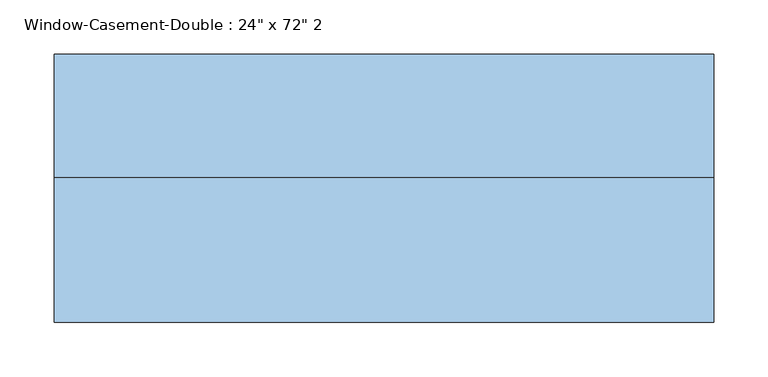
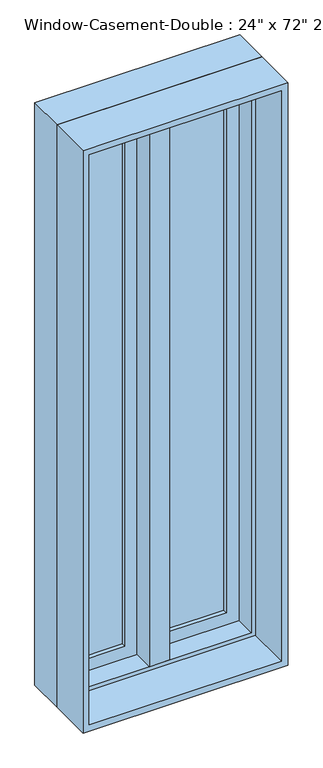
"""IFC4 building model written with IfcOpenShell, lengths in millimetres: window geometry."""

from ifc_helpers import new_model, si_unit, frame, origin, place, context, project, spatial, polyline, outline, extrude, faceted_brep, source, transform, mapped, element, save


def window_0389f97f(model_context):
    return source(origin(), model_context, "Body", "SolidModel", [
        faceted_brep([(9.525, 133.35, 2730.5), (-9.525, 133.35, 2730.5), (-9.525, 82.55, 2730.5), (9.525, 82.55, 2730.5), (9.525, 133.35, 927.1), (9.525, 82.55, 927.1), (-9.525, 82.55, 927.1), (-9.525, 133.35, 927.1), (-9.525, 82.55, 946.15), (-9.525, 82.55, 2711.45), (-30.1625, 82.55, 946.15), (-30.1625, 82.55, 2711.45), (-30.1625, 19.05, 946.15), (-30.1625, 19.05, 2711.45), (30.1625, 19.05, 946.15), (30.1625, 19.05, 2711.45), (30.1625, 82.55, 946.15), (30.1625, 82.55, 2711.45), (9.525, 82.55, 946.15), (9.525, 82.55, 2711.45)], [[[0, 1, 2, 3]], [[4, 5, 6, 7]], [[1, 0, 4, 7]], [[2, 1, 7, 6, 8, 9]], [[9, 8, 10, 11]], [[11, 10, 12, 13]], [[13, 12, 14, 15]], [[15, 14, 16, 17]], [[17, 16, 18, 19]], [[0, 3, 19, 18, 5, 4]], [[18, 8, 6, 5]], [[9, 19, 3, 2]], [[8, 18, 16, 14, 12, 10]], [[19, 9, 11, 13, 15, 17]]]),
        extrude(outline(polyline([(-66.675, 114.3), (-66.675, 107.95), (-234.95, 107.95), (-234.95, 114.3), (-66.675, 114.3)])), frame((0.0, 0.0, 984.25), z_axis=(0.0, 0.0, 1.0), x_axis=(1.0, 0.0, 0.0)), (0.0, 0.0, 1.0), 1689.1),
        extrude(outline(polyline([(-234.95, 95.25), (-234.95, 101.6), (-66.675, 101.6), (-66.675, 95.25), (-234.95, 95.25)])), frame((0.0, 0.0, 984.25), z_axis=(0.0, 0.0, 1.0), x_axis=(1.0, 0.0, 0.0)), (0.0, 0.0, 1.0), 1689.1),
        extrude(outline(polyline([(234.95, 114.3), (234.95, 107.95), (66.675, 107.95), (66.675, 114.3), (234.95, 114.3)])), frame((0.0, 0.0, 984.25), z_axis=(0.0, 0.0, 1.0), x_axis=(1.0, 0.0, 0.0)), (0.0, 0.0, 1.0), 1689.1),
        extrude(outline(polyline([(66.675, 95.25), (66.675, 101.6), (234.95, 101.6), (234.95, 95.25), (66.675, 95.25)])), frame((0.0, 0.0, 984.25), z_axis=(0.0, 0.0, 1.0), x_axis=(1.0, 0.0, 0.0)), (0.0, 0.0, 1.0), 1689.1),
        extrude(outline(polyline([(2730.5, -292.1), (927.1, -292.1), (927.1, -9.525), (2730.5, -9.525), (2730.5, -292.1)]), holes=[polyline([(2673.35, -66.675), (984.25, -66.675), (984.25, -234.95), (2673.35, -234.95), (2673.35, -66.675)])]), frame((0.0, 82.55, 0.0), z_axis=(0.0, 1.0, 0.0), x_axis=(0.0, 0.0, 1.0)), (0.0, 0.0, 1.0), 44.45),
        extrude(outline(polyline([(927.1, 292.1), (2730.5, 292.1), (2730.5, 9.525), (927.1, 9.525), (927.1, 292.1)]), holes=[polyline([(984.25, 66.675), (2673.35, 66.675), (2673.35, 234.95), (984.25, 234.95), (984.25, 66.675)])]), frame((0.0, 82.55, 0.0), z_axis=(0.0, 1.0, 0.0), x_axis=(0.0, 0.0, 1.0)), (0.0, 0.0, 1.0), 44.45),
        extrude(outline(polyline([(2743.2, -304.8), (914.4, -304.8), (914.4, 304.8), (2743.2, 304.8), (2743.2, -304.8)]), holes=[polyline([(2724.15, 285.75), (933.45, 285.75), (933.45, -285.75), (2724.15, -285.75), (2724.15, 285.75)])]), frame((0.0, -114.3, 0.0), z_axis=(0.0, 1.0, 0.0), x_axis=(0.0, 0.0, 1.0)), (0.0, 0.0, 1.0), 133.35),
        faceted_brep([(273.05, 82.55, 2711.45), (273.05, 19.05, 2711.45), (-273.05, 19.05, 2711.45), (-273.05, 82.55, 2711.45), (292.1, 133.35, 2730.5), (292.1, 82.55, 2730.5), (-292.1, 82.55, 2730.5), (-292.1, 133.35, 2730.5), (304.8, 19.05, 2743.2), (304.8, 133.35, 2743.2), (-304.8, 133.35, 2743.2), (-304.8, 19.05, 2743.2), (-273.05, 19.05, 946.15), (-273.05, 82.55, 946.15), (-292.1, 82.55, 927.1), (-292.1, 133.35, 927.1), (-304.8, 133.35, 914.4), (-304.8, 19.05, 914.4), (273.05, 19.05, 946.15), (273.05, 82.55, 946.15), (292.1, 82.55, 927.1), (292.1, 133.35, 927.1), (304.8, 133.35, 914.4), (304.8, 19.05, 914.4)], [[[0, 1, 2, 3]], [[4, 5, 6, 7]], [[8, 9, 10, 11]], [[3, 2, 12, 13]], [[7, 6, 14, 15]], [[11, 10, 16, 17]], [[13, 12, 18, 19]], [[15, 14, 20, 21]], [[17, 16, 22, 23]], [[11, 17, 23, 8], [1, 18, 12, 2]], [[19, 18, 1, 0]], [[5, 20, 14, 6], [3, 13, 19, 0]], [[21, 20, 5, 4]], [[23, 22, 9, 8]], [[9, 22, 16, 10], [7, 15, 21, 4]]]),
    ])


if __name__ == "__main__":
    model = new_model("IFC4")
    model_context = context("Model", 3, world=origin())
    ifc_project = project(units=[si_unit("LENGTHUNIT", "METRE", prefix="MILLI")], contexts=[model_context])
    site = spatial("IfcSite", under=ifc_project)
    building = spatial("IfcBuilding", under=site)
    placement = place(None, origin())
    window_shape = window_0389f97f(model_context)
    element("IfcWindow", 1, ObjectType="Window-Casement-Double : 24\" x 72\" 2", at=placement, inside=building, context=model_context, shape_type="MappedRepresentation", body=[
        mapped(window_shape, transform((0.0, 0.0, 0.0), x_axis=(1.0, 0.0, 0.0), y_axis=(0.0, 1.0, 0.0), z_axis=(0.0, 0.0, 1.0))),
    ])
    save(model, "model.ifc")

# Revit data of these elements
# Type "Window-Casement-Double : 24\" x 72\" 2"
#   Type Mark = "28"
#   Fire Rating = "0.5h"
#   Assembly Code = "B2020100"
#   Analytic Construction = "Double glazing - domestic"
#   Frame Extension [instance default] = 0' - 0 1/4"
#   Window Inset [instance default] = 0' - 0"
#   Wall Thickness [instance default] = 0' - 6"
#   Interior Wall Closure [instance default] = 0' - 2 1/4"
#   Half Width = 1' - 0"
#   Visual Light Transmittance = 0.81
#   Thermal Resistance (R) = 1.8146 (h·ft²·°F)/BTU
#   Solar Heat Gain Coefficient = 0.76
#   Rough Width = 2' - 0 1/2"
#   Rough Height = 6' - 0 1/2"
#   Height = 6' - 0"
#   Heat Transfer Coefficient (U) = 0.5511 BTU/(h·ft²·°F)
#   Exterior Wall Closure [instance default] = 0' - 1 1/4"
#   Extension Jamb [instance default] = 0' - 2 1/4"
#   Default Sill Height = 3' - 0"
#   Width = 2' - 0"
#   Muntin Visibility = yes
#   Interior Trim Visibility [instance default] = yes
#   Exterior Trim Visibility [instance default] = yes
#   Extension Jamb Visibility [instance default] = yes
#   Interior Trim Material = Wood - Stained
#   Muntin Pattern = Muntin Pattern_2x2 : Muntin Pattern_2x2
#   Interior Trim = Trim-Window-Interior-Flat : Picture Frame
#   Interior Frame Material = Wood - Stained
#   Glass Panel Material = Glass
#   Exterior Trim Material = Clad - White
#   Exterior Trim = Trim-Window-Exterior-Flat : with Sill
#   Exterior Frame Material = Clad - White
#   Wall Closure = (empty or 0)
# Element 1 (IfcWindow, "Window-Casement-Double : 24\" x 72\" 2")
#   Wall Thickness = 0' - 9"
#   Extension Jamb = 0' - 5 1/4"
#   Materials on its faces: "Wood - Stained", "Glass", "Clad - White"
# Materials
#   "Wood - Stained": class "Wood", colour RGB 224 178 126, transparency 0, Cost = 0
#   "Glass": class "Glass", colour RGB 0 128 192, transparency 0.75, Description = "Soda Lime Glass", Cost = 0
#   "Clad - White": class "Wood", colour RGB 242 242 238, transparency 0, Cost = 0
